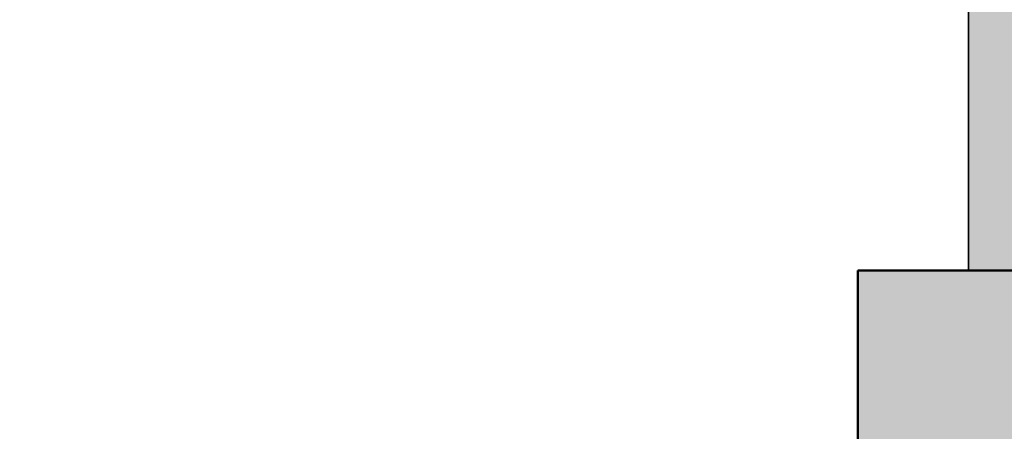
# Model space of a CAD drawing. Units: inches. Extents: x 1998 to 2588, y 1139 to 1977.
# Tile 52 of 134: x 2282 to 2344, y 1637 to 1663. Entities that reach past the tile are written whole.
import ezdxf

# ---------------------------------------------------------------- set-up
doc = ezdxf.new("R2010")
doc.units = ezdxf.units.IN
for name, color, linetype, lineweight in [('A-COLS-PATT', 250, 'Continuous', 13), ('A-WALL-PATT', 252, 'Continuous', 13), ('COLUMN', 10, 'Continuous', 50), ('WALL', 200, 'Continuous', 35)]:
    doc.layers.add(name, color=color, linetype=linetype, lineweight=lineweight)

msp = doc.modelspace()

# ---------------------------------------------------------------- hatches: boundary and pattern name
at = {"layer": 'A-COLS-PATT'}
h = msp.add_hatch(color=256, dxfattribs=at)
h.dxf.hatch_style = 1
h.paths.add_polyline_path([(2099.4125, 1888.7324), (2087.9729, 1888.7324), (2087.9729, 1868.3278), (2099.4125, 1868.3278)])
h.paths.add_polyline_path([(2234.4125, 1888.7324), (2222.9729, 1888.7324), (2222.9729, 1868.3278), (2234.4125, 1868.3278)])
h.paths.add_polyline_path([(2341.4729, 1886.637), (2330.0332, 1886.637), (2330.0332, 1866.2324), (2341.4729, 1866.2324)])
h.paths.add_polyline_path([(2507.8006, 1882.7324), (2487.396, 1882.7324), (2487.396, 1871.2927), (2507.8006, 1871.2927)])
h.paths.add_polyline_path([(2510.9729, 1766.672), (2490.5682, 1766.672), (2490.5682, 1755.2324), (2510.9729, 1755.2324)])
h.paths.add_polyline_path([(2345.9729, 1759.7324), (2334.5332, 1759.7324), (2334.5332, 1739.3278), (2345.9729, 1739.3278)])
h.paths.add_polyline_path([(2234.4125, 1774.3318), (2222.9729, 1774.3318), (2222.9729, 1753.9272), (2234.4125, 1753.9272)])
h.paths.add_polyline_path([(2099.4125, 1775.637), (2087.9729, 1775.637), (2087.9729, 1755.2324), (2099.4125, 1755.2324)])
h.paths.add_polyline_path([(2098.0956, 1593.7241), (2077.691, 1593.7241), (2077.691, 1582.2845), (2098.0956, 1582.2845)])
h.paths.add_polyline_path([(2227.4729, 1604.637), (2216.0332, 1604.637), (2216.0332, 1584.2324), (2227.4729, 1584.2324)])
h.paths.add_polyline_path([(2345.9729, 1647.5211), (2334.5332, 1647.5211), (2334.5332, 1627.1165), (2345.9729, 1627.1165)])
h.paths.add_polyline_path([(2522.3775, 1641.2324), (2501.9729, 1641.2324), (2501.9729, 1629.7927), (2522.3775, 1629.7927)])
h.paths.add_polyline_path([(2522.3775, 1480.7324), (2501.9729, 1480.7324), (2501.9729, 1469.2927), (2522.3775, 1469.2927)])
h.paths.add_polyline_path([(2345.9729, 1488.5616), (2334.5332, 1488.5616), (2334.5332, 1468.1569), (2345.9729, 1468.1569)])
h.paths.add_polyline_path([(2234.4125, 1486.137), (2227.4729, 1486.137), (2227.4729, 1465.7324), (2234.4125, 1465.7324)])
h.paths.add_polyline_path([(2227.4729, 1486.137), (2222.9729, 1486.137), (2222.9729, 1465.7324), (2227.4729, 1465.7324)])
h.paths.add_polyline_path([(2108.3775, 1470.2324), (2087.9729, 1470.2324), (2087.9729, 1458.7927), (2108.3775, 1458.7927)])
h.paths.add_polyline_path([(2096.9729, 1365.5012), (2087.9729, 1365.5012), (2087.9729, 1345.0966), (2096.9729, 1345.0966)])
h.paths.add_polyline_path([(2087.9729, 1365.5012), (2085.5332, 1365.5012), (2085.5332, 1345.0966), (2087.9729, 1345.0966)])
h.paths.add_polyline_path([(2234.4125, 1285.137), (2222.9729, 1285.137), (2222.9729, 1264.7324), (2234.4125, 1264.7324)])
h.paths.add_polyline_path([(2345.9729, 1285.137), (2334.5332, 1285.137), (2334.5332, 1264.7324), (2345.9729, 1264.7324)])
h.paths.add_polyline_path([(2503.1458, 1240.172), (2482.7412, 1240.172), (2482.7412, 1228.7324), (2503.1458, 1228.7324)])
h.paths.add_polyline_path([(2510.9729, 1369.172), (2490.5682, 1369.172), (2490.5682, 1357.7324), (2510.9729, 1357.7324)])
at = {"layer": 'A-WALL-PATT'}
h = msp.add_hatch(color=256, dxfattribs=at)
h.dxf.hatch_style = 1
h.paths.add_polyline_path([(2527.4729, 1362.2324), (2510.9729, 1362.2324), (2510.9729, 1357.7324), (2518.4729, 1357.7324), (2518.4729, 1237.7324), (2503.1458, 1237.7324), (2503.1458, 1228.7324), (2527.4729, 1228.7324)])
h.paths.add_polyline_path([(2490.5682, 1362.2324), (2398.4729, 1362.2324), (2398.4729, 1357.7324), (2490.5682, 1357.7324)])
h.paths.add_polyline_path([(2224.9729, 1264.7324), (2222.9729, 1264.7324), (2222.9729, 1232.4125), (2341.4729, 1232.4125), (2341.4729, 1234.4125), (2224.9729, 1234.4125)])
h.paths.add_polyline_path([(2334.5332, 1273.7324), (2264.7638, 1273.7324), (2264.7638, 1269.5611, -0.043659), (2264.3413, 1264.7324), (2334.5332, 1264.7324)])
h.paths.add_polyline_path([(2236.9551, 1273.7324), (2234.4125, 1273.7324), (2234.4125, 1264.7324), (2236.9551, 1264.7324), (2236.9551, 1269.5611)])
h.paths.add_polyline_path([(2222.9729, 1293.2324), (2096.9729, 1293.2324), (2096.9729, 1345.0966), (2087.9729, 1345.0966), (2087.9729, 1284.2324), (2222.9729, 1284.2324), (2222.9729, 1285.137)])
h.paths.add_polyline_path([(2096.9729, 1458.7927), (2087.9729, 1458.7927), (2087.9729, 1417.7324), (2087.9729, 1413.2324), (2096.9729, 1413.2324), (2096.9729, 1417.7324)])
h.paths.add_polyline_path([(2096.9729, 1413.2324), (2087.9729, 1413.2324), (2087.9729, 1365.5012), (2096.9729, 1365.5012), (2096.9729, 1369.3358)])
h.paths.add_polyline_path([(2186.2943, 1417.7324), (2138.6074, 1417.7324), (2096.9729, 1417.7324), (2096.9729, 1413.2324), (2138.6074, 1413.2324), (2186.2943, 1413.2324)])
h.paths.add_polyline_path([(2181.4729, 1465.7324), (2176.9729, 1465.7324), (2176.9729, 1451.6434), (2181.4729, 1451.6434)])
h.paths.add_polyline_path([(2181.4729, 1422.1664), (2176.9729, 1422.1664), (2176.9729, 1417.7324), (2181.4729, 1417.7324)])
h.paths.add_polyline_path([(2063.9729, 1465.7324), (2087.9729, 1465.7324), (2087.9729, 1470.2324), (2059.4729, 1470.2324), (2059.4729, 1413.2324), (2087.9729, 1413.2324), (2087.9729, 1417.7324), (2063.9729, 1417.7324)])
h.paths.add_polyline_path([(2181.4729, 1755.2324), (2176.9729, 1755.2324), (2176.9729, 1748.6798), (2177.0513, 1748.6798), (2181.4729, 1748.6798)])
h.paths.add_polyline_path([(2227.4729, 1707.2324), (2220.4647, 1707.2324), (2220.4647, 1702.7324), (2222.9729, 1702.7324), (2222.9729, 1604.637), (2227.4729, 1604.637)])
h.paths.add_polyline_path([(2114.9729, 1702.7324), (2105.9729, 1702.7324), (2105.9729, 1628.4781, -0.0318759), (2110.1012, 1628.7416), (2114.9729, 1628.7416)])
h.paths.add_polyline_path([(2345.9729, 1739.3278), (2341.4729, 1739.3278), (2341.4729, 1647.5211), (2345.9729, 1647.5211)])
h.paths.add_polyline_path([(2350.6273, 1641.2324), (2345.9729, 1641.2324), (2345.9729, 1636.7324), (2350.6273, 1636.7324), (2350.6273, 1639.8729)])
h.paths.add_polyline_path([(2501.9729, 1641.2324), (2407.9729, 1641.2324), (2392.5005, 1641.2324), (2392.5005, 1639.8729), (2392.5005, 1636.7324), (2501.9729, 1636.7324)])
h.paths.add_polyline_path([(2510.9729, 1755.2324), (2501.9729, 1755.2324), (2501.9729, 1641.2324), (2510.9729, 1641.2324)])
h.paths.add_polyline_path([(2549.1786, 1641.2324), (2522.3775, 1641.2324), (2522.3775, 1636.7324), (2540.1786, 1636.7324), (2540.1786, 1480.7324), (2522.3775, 1480.7324), (2522.3775, 1476.2324), (2549.1786, 1476.2324)])
h.paths.add_polyline_path([(2498.1786, 1594.7324), (2407.9729, 1594.7324), (2407.9729, 1585.7324), (2416.9729, 1585.7324), (2489.1786, 1585.7324), (2489.1786, 1531.7324), (2416.9729, 1531.7324), (2407.9729, 1531.7324), (2407.9729, 1522.7324), (2498.1786, 1522.7324)])
h.paths.add_polyline_path([(2351.6437, 1480.7324), (2345.9729, 1480.7324), (2345.9729, 1476.2324), (2351.6437, 1476.2324), (2351.6437, 1477.5919)])
h.paths.add_polyline_path([(2501.9729, 1480.7324), (2498.1786, 1480.7324), (2407.9729, 1480.7324), (2393.5168, 1480.7324), (2393.5168, 1477.5919), (2393.5168, 1476.2324), (2501.9729, 1476.2324)])

# ---------------------------------------------------------------- linework, layer by layer
at = {"layer": 'COLUMN'}
msp.add_lwpolyline([(2334.5332, 1647.5211), (2345.9729, 1647.5211), (2345.9729, 1627.1165), (2334.5332, 1627.1165)], close=True, dxfattribs=at)
at = {"layer": 'WALL'}
msp.add_line((2341.4729, 1739.3278), (2341.4729, 1647.5211), dxfattribs=at)

doc.saveas('drawing.dxf')
